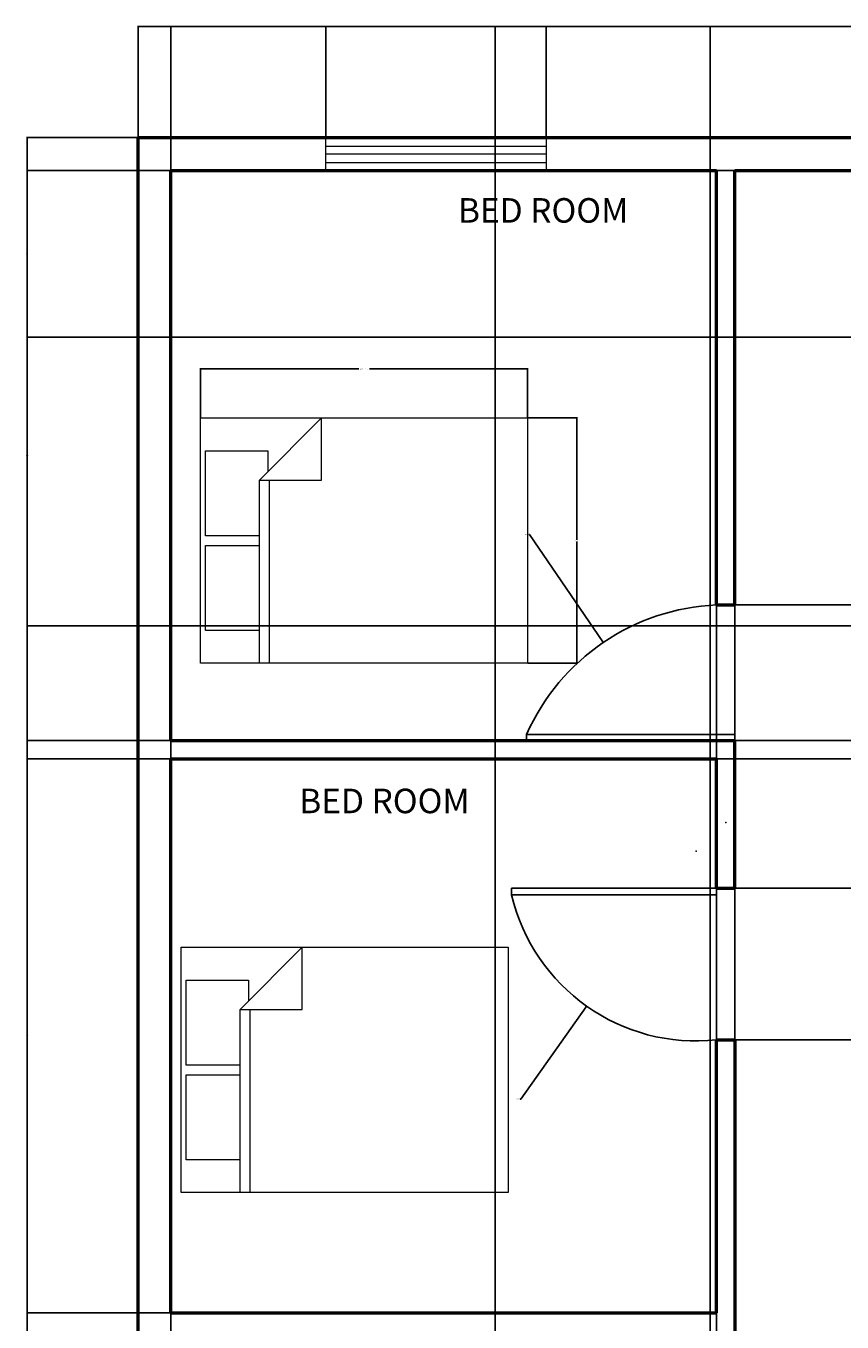
# Model space of a CAD drawing. Units: inches. Extents: x 2907 to 3328, y 1715 to 2286.
# Tile 3 of 5: x 2907 to 3107, y 1969 to 2286. Entities that reach past the tile are written whole.
import ezdxf

# ---------------------------------------------------------------- set-up
doc = ezdxf.new("R2010")
doc.units = ezdxf.units.IN
for name, color, linetype, lineweight in [('A-ANNO-DIMS', 2, 'Continuous', 18), ('A-AREA-IDEN', 7, 'Continuous', 25), ('A-DOOR', 3, 'Continuous', 25), ('A-FURN', 8, 'Continuous', 18), ('A-GLAZ', 4, 'Continuous', 18), ('A-WALL', 7, 'Continuous', 50)]:
    doc.layers.add(name, color=color, linetype=linetype, lineweight=lineweight)
doc.styles.get("Standard").update_dxf_attribs({"font": 'arial.ttf'})
doc.dimstyles.get("Standard").update_dxf_attribs({"dimtxt": 0.18, "dimasz": 0.18, "dimexe": 0.18, "dimexo": 0.0625, "dimgap": 0.09, "dimtad": 0, "dimtih": 1, "dimtoh": 1, "dimdec": 4, "dimzin": 0, "dimdsep": 46, "dimtxsty": 'Standard', "dimcen": 0.09, "dimadec": 0, "dimazin": 0, "dimtfac": 1, "dimtdec": 4, "dimtofl": 0, "dimtmove": 0, "dimatfit": 3, "dimfxl": 1, "dimtolj": 1, "dimtzin": 0, "dimarcsym": 0})

# ---------------------------------------------------------------- blocks, each defined once
blk = doc.blocks.new('Bed - Queen')
for p, q in [((0, -80.00003), (0, 0)), ((0, 0), (59.99999, 0)), ((59.99999, 0), (59.99999, -80.00003)), ((7.99999, -1.2), (28.79998, -1.2)), ((7.99999, -14.4), (7.99999, -1.2)), ((28.79998, -1.2), (28.79998, -14.4)), ((31.19999, -1.2), (51.99999, -1.2)), ((31.19999, -14.4), (31.19999, -1.2)), ((51.99999, -1.2), (51.99999, -16.4)), ((0, -14.4), (44.8, -14.4)), ((59.99999, -29.6), (44.8, -14.4)), ((44.8, -14.4), (44.8, -29.6)), ((44.8, -16.8), (0, -16.8)), ((51.99999, -16.4), (46.79936, -16.4)), ((44.8, -29.6), (59.99999, -29.6)), ((59.99999, -80.00003), (0, -80.00003))]:
    blk.add_line(p, q)
blk = doc.blocks.new('*D5')
at = {"layer": 'A-ANNO-DIMS', "color": 0, "lineweight": -2, "transparency": 16777216}
for p, q in [((2949.87, 2190.31), (2949.87, 2202.43)), ((2950.05, 2202.25), (2988.57, 2202.25)), ((3029.69, 2202.25), (2991.18, 2202.25)), ((3029.87, 2190.31), (3029.87, 2202.43))]:
    blk.add_line(p, q, dxfattribs=at)
at = {"layer": 'A-ANNO-DIMS', "color": 0, "transparency": 16777216}
for points in [[(2950.05, 2202.28), (2950.05, 2202.22), (2949.87, 2202.25)], [(3029.69, 2202.28), (3029.69, 2202.22), (3029.87, 2202.25)]]:
    blk.add_solid(points, dxfattribs=at)
at = {"layer": 'Defpoints', "color": 0, "transparency": 16777216}
for p in [(2949.87, 2202.25), (2949.87, 2190.25), (3029.87, 2190.25)]:
    blk.add_point(p, dxfattribs=at)
at = {"layer": 'A-ANNO-DIMS', "color": 0, "transparency": 16777216, "insert": (2989.87, 2202.25), "char_height": 0.18, "attachment_point": 5}
blk.add_mtext('\\A1;QUEEN BED 80 TYP.', dxfattribs=at)
blk = doc.blocks.new('*D6')
at = {"layer": 'A-ANNO-DIMS', "color": 0, "lineweight": -2, "transparency": 16777216}
for p, q in [((3029.94, 2190.25), (3042.05, 2190.25)), ((3041.87, 2190.07), (3041.87, 2160.43)), ((3041.87, 2130.43), (3041.87, 2160.07)), ((3029.94, 2130.25), (3042.05, 2130.25))]:
    blk.add_line(p, q, dxfattribs=at)
at = {"layer": 'A-ANNO-DIMS', "color": 0, "transparency": 16777216}
for points in [[(3041.84, 2190.07), (3041.9, 2190.07), (3041.87, 2190.25)], [(3041.84, 2130.43), (3041.9, 2130.43), (3041.87, 2130.25)]]:
    blk.add_solid(points, dxfattribs=at)
at = {"layer": 'Defpoints', "color": 0, "transparency": 16777216}
for p in [(3029.87, 2190.25), (3041.87, 2190.25), (3029.87, 2130.25)]:
    blk.add_point(p, dxfattribs=at)
at = {"layer": 'A-ANNO-DIMS', "color": 0, "transparency": 16777216, "insert": (3041.87, 2160.25), "char_height": 0.18, "attachment_point": 5}
blk.add_mtext('\\A1;60 TYP.', dxfattribs=at)
blk = doc.blocks.new('*D13')
at = {"layer": 'A-ANNO-DIMS', "color": 0, "lineweight": -2, "transparency": 16777216}
for p, q in [((2934.59, 2258.89), (2934.59, 2286.16)), ((3300.59, 2258.89), (3300.59, 2286.16)), ((2934.77, 2285.98), (3117.3, 2285.98)), ((3300.41, 2285.98), (3117.88, 2285.98))]:
    blk.add_line(p, q, dxfattribs=at)
at = {"layer": 'A-ANNO-DIMS', "color": 0, "transparency": 16777216}
for points in [[(2934.77, 2286.01), (2934.77, 2285.95), (2934.59, 2285.98)], [(3300.41, 2286.01), (3300.41, 2285.95), (3300.59, 2285.98)]]:
    blk.add_solid(points, dxfattribs=at)
at = {"layer": 'Defpoints', "color": 0, "transparency": 16777216}
for p in [(3300.59, 2285.98), (2934.59, 2258.83), (3300.59, 2258.83)]:
    blk.add_point(p, dxfattribs=at)
at = {"layer": 'A-ANNO-DIMS', "color": 0, "transparency": 16777216, "insert": (3117.59, 2285.98), "char_height": 0.18, "attachment_point": 5}
blk.add_mtext('\\A1;366', dxfattribs=at)
blk = doc.blocks.new('*D14')
at = {"layer": 'A-ANNO-DIMS', "color": 0, "lineweight": -2, "transparency": 16777216}
for p, q in [((2934.53, 2258.83), (2907.26, 2258.83)), ((2907.44, 2258.65), (2907.44, 2001.01)), ((2907.44, 1743.01), (2907.44, 2000.65)), ((2934.53, 1742.83), (2907.26, 1742.83))]:
    blk.add_line(p, q, dxfattribs=at)
at = {"layer": 'A-ANNO-DIMS', "color": 0, "transparency": 16777216}
for points in [[(2907.41, 2258.65), (2907.47, 2258.65), (2907.44, 2258.83)], [(2907.41, 1743.01), (2907.47, 1743.01), (2907.44, 1742.83)]]:
    blk.add_solid(points, dxfattribs=at)
at = {"layer": 'Defpoints', "color": 0, "transparency": 16777216}
for p in [(2907.44, 2258.83), (2934.59, 2258.83), (2934.59, 1742.83)]:
    blk.add_point(p, dxfattribs=at)
at = {"layer": 'A-ANNO-DIMS', "color": 0, "transparency": 16777216, "insert": (2907.44, 2000.83), "char_height": 0.18, "attachment_point": 5}
blk.add_mtext('\\A1;516', dxfattribs=at)
blk = doc.blocks.new('*D16')
at = {"layer": 'A-ANNO-DIMS', "color": 0, "lineweight": -2, "transparency": 16777216}
for p, q in [((2942.59, 2250.77), (2942.59, 1715.5)), ((3076.09, 2250.77), (3076.09, 1715.5)), ((2942.77, 1715.68), (3008.95, 1715.68)), ((3075.91, 1715.68), (3009.73, 1715.68))]:
    blk.add_line(p, q, dxfattribs=at)
at = {"layer": 'A-ANNO-DIMS', "color": 0, "transparency": 16777216}
for points in [[(2942.77, 1715.71), (2942.77, 1715.65), (2942.59, 1715.68)], [(3075.91, 1715.71), (3075.91, 1715.65), (3076.09, 1715.68)]]:
    blk.add_solid(points, dxfattribs=at)
at = {"layer": 'Defpoints', "color": 0, "transparency": 16777216}
for p in [(2942.59, 2250.83), (3076.09, 2250.83), (3076.09, 1715.68)]:
    blk.add_point(p, dxfattribs=at)
at = {"layer": 'A-ANNO-DIMS', "color": 0, "transparency": 16777216, "insert": (3009.34, 1715.68), "char_height": 0.18, "attachment_point": 5}
blk.add_mtext('\\A1;133.5', dxfattribs=at)
blk = doc.blocks.new('*D17')
at = {"layer": 'A-ANNO-DIMS', "color": 0, "lineweight": -2, "transparency": 16777216}
for p, q in [((3080.59, 2250.77), (3080.59, 1715.5)), ((3192.09, 2250.77), (3192.09, 1715.5)), ((3080.77, 1715.68), (3135.95, 1715.68)), ((3191.91, 1715.68), (3136.73, 1715.68))]:
    blk.add_line(p, q, dxfattribs=at)
at = {"layer": 'A-ANNO-DIMS', "color": 0, "transparency": 16777216}
for points in [[(3080.77, 1715.71), (3080.77, 1715.65), (3080.59, 1715.68)], [(3191.91, 1715.71), (3191.91, 1715.65), (3192.09, 1715.68)]]:
    blk.add_solid(points, dxfattribs=at)
at = {"layer": 'Defpoints', "color": 0, "transparency": 16777216}
for p in [(3080.59, 2250.83), (3192.09, 2250.83), (3192.09, 1715.68)]:
    blk.add_point(p, dxfattribs=at)
at = {"layer": 'A-ANNO-DIMS', "color": 0, "transparency": 16777216, "insert": (3136.34, 1715.68), "char_height": 0.18, "attachment_point": 5}
blk.add_mtext('\\A1;111.5', dxfattribs=at)
blk = doc.blocks.new('*D19')
at = {"layer": 'A-ANNO-DIMS', "color": 0, "lineweight": -2, "transparency": 16777216}
for p, q in [((2934.59, 2258.89), (2934.59, 2286.16)), ((2980.47, 2258.89), (2980.47, 2286.16)), ((2934.77, 2285.98), (2957.13, 2285.98)), ((2980.29, 2285.98), (2957.93, 2285.98))]:
    blk.add_line(p, q, dxfattribs=at)
at = {"layer": 'A-ANNO-DIMS', "color": 0, "transparency": 16777216}
for points in [[(2934.77, 2286.01), (2934.77, 2285.95), (2934.59, 2285.98)], [(2980.29, 2286.01), (2980.29, 2285.95), (2980.47, 2285.98)]]:
    blk.add_solid(points, dxfattribs=at)
at = {"layer": 'Defpoints', "color": 0, "transparency": 16777216}
for p in [(2980.47, 2285.98), (2934.59, 2258.83), (2980.47, 2258.83)]:
    blk.add_point(p, dxfattribs=at)
at = {"layer": 'A-ANNO-DIMS', "color": 0, "transparency": 16777216, "insert": (2957.53, 2285.98), "char_height": 0.18, "attachment_point": 5}
blk.add_mtext('\\A1;45.88', dxfattribs=at)
blk = doc.blocks.new('*D20')
at = {"layer": 'A-ANNO-DIMS', "color": 0, "lineweight": -2, "transparency": 16777216}
for p, q in [((2980.47, 2258.89), (2980.47, 2286.16)), ((3034.37, 2258.89), (3034.37, 2286.16)), ((2980.65, 2285.98), (3007.09, 2285.98)), ((3034.19, 2285.98), (3007.74, 2285.98))]:
    blk.add_line(p, q, dxfattribs=at)
at = {"layer": 'A-ANNO-DIMS', "color": 0, "transparency": 16777216}
for points in [[(2980.65, 2286.01), (2980.65, 2285.95), (2980.47, 2285.98)], [(3034.19, 2286.01), (3034.19, 2285.95), (3034.37, 2285.98)]]:
    blk.add_solid(points, dxfattribs=at)
at = {"layer": 'Defpoints', "color": 0, "transparency": 16777216}
for p in [(3034.37, 2285.98), (2980.47, 2258.83), (3034.37, 2258.83)]:
    blk.add_point(p, dxfattribs=at)
at = {"layer": 'A-ANNO-DIMS', "color": 0, "transparency": 16777216, "insert": (3007.42, 2285.98), "char_height": 0.18, "attachment_point": 5}
blk.add_mtext('\\A1;53.9', dxfattribs=at)
blk = doc.blocks.new('*D25')
at = {"layer": 'A-ANNO-DIMS', "color": 0, "lineweight": -2, "transparency": 16777216}
for p, q in [((2942.53, 2250.83), (2907.26, 2250.83)), ((2907.44, 2250.65), (2907.44, 2181.26)), ((2907.44, 2111.51), (2907.44, 2180.9)), ((2942.53, 2111.33), (2907.26, 2111.33))]:
    blk.add_line(p, q, dxfattribs=at)
at = {"layer": 'A-ANNO-DIMS', "color": 0, "transparency": 16777216}
for points in [[(2907.41, 2250.65), (2907.47, 2250.65), (2907.44, 2250.83)], [(2907.41, 2111.51), (2907.47, 2111.51), (2907.44, 2111.33)]]:
    blk.add_solid(points, dxfattribs=at)
at = {"layer": 'Defpoints', "color": 0, "transparency": 16777216}
for p in [(2907.44, 2250.83), (2942.59, 2250.83), (2942.59, 2111.33)]:
    blk.add_point(p, dxfattribs=at)
at = {"layer": 'A-ANNO-DIMS', "color": 0, "transparency": 16777216, "insert": (2907.44, 2181.08), "char_height": 0.18, "attachment_point": 5}
blk.add_mtext('\\A1;139.5', dxfattribs=at)
blk = doc.blocks.new('*D26')
at = {"layer": 'A-ANNO-DIMS', "color": 0, "lineweight": -2, "transparency": 16777216}
for p, q in [((2942.53, 2106.83), (2907.26, 2106.83)), ((2907.44, 2106.65), (2907.44, 2039.26)), ((2907.44, 1971.51), (2907.44, 2038.9)), ((2942.53, 1971.33), (2907.26, 1971.33))]:
    blk.add_line(p, q, dxfattribs=at)
at = {"layer": 'A-ANNO-DIMS', "color": 0, "transparency": 16777216}
for points in [[(2907.41, 2106.65), (2907.47, 2106.65), (2907.44, 2106.83)], [(2907.41, 1971.51), (2907.47, 1971.51), (2907.44, 1971.33)]]:
    blk.add_solid(points, dxfattribs=at)
at = {"layer": 'Defpoints', "color": 0, "transparency": 16777216}
for p in [(2907.44, 2106.83), (2942.59, 2106.83), (2942.59, 1971.33)]:
    blk.add_point(p, dxfattribs=at)
at = {"layer": 'A-ANNO-DIMS', "color": 0, "transparency": 16777216, "insert": (2907.44, 2039.08), "char_height": 0.18, "attachment_point": 5}
blk.add_mtext('\\A1;135.5', dxfattribs=at)
blk = doc.blocks.new('*D31')
at = {"layer": 'A-ANNO-DIMS', "color": 0, "lineweight": -2, "transparency": 16777216}
for p, q in [((2942.59, 1912.39), (2942.59, 2286.16)), ((3021.96, 1912.39), (3021.96, 2286.16)), ((2942.77, 2285.98), (2981.88, 2285.98)), ((3021.78, 2285.98), (2982.67, 2285.98))]:
    blk.add_line(p, q, dxfattribs=at)
at = {"layer": 'A-ANNO-DIMS', "color": 0, "transparency": 16777216}
for points in [[(2942.77, 2286.01), (2942.77, 2285.95), (2942.59, 2285.98)], [(3021.78, 2286.01), (3021.78, 2285.95), (3021.96, 2285.98)]]:
    blk.add_solid(points, dxfattribs=at)
at = {"layer": 'Defpoints', "color": 0, "transparency": 16777216}
for p in [(3021.96, 2285.98), (2942.59, 1912.33), (3021.96, 1912.33)]:
    blk.add_point(p, dxfattribs=at)
at = {"layer": 'A-ANNO-DIMS', "color": 0, "transparency": 16777216, "insert": (2982.27, 2285.98), "char_height": 0.18, "attachment_point": 5}
blk.add_mtext('\\A1;79.37', dxfattribs=at)
blk = doc.blocks.new('*D34')
at = {"layer": 'A-ANNO-DIMS', "color": 0, "lineweight": -2, "transparency": 16777216}
for p, q in [((3074.5, 1778.89), (3074.5, 2286.16)), ((3131.97, 1778.89), (3131.97, 2286.16)), ((3074.68, 2285.98), (3102.84, 2285.98)), ((3131.79, 2285.98), (3103.63, 2285.98))]:
    blk.add_line(p, q, dxfattribs=at)
at = {"layer": 'A-ANNO-DIMS', "color": 0, "transparency": 16777216}
for points in [[(3074.68, 2286.01), (3074.68, 2285.95), (3074.5, 2285.98)], [(3131.79, 2286.01), (3131.79, 2285.95), (3131.97, 2285.98)]]:
    blk.add_solid(points, dxfattribs=at)
at = {"layer": 'Defpoints', "color": 0, "transparency": 16777216}
for p in [(3131.97, 2285.98), (3074.5, 1778.83), (3131.97, 1778.83)]:
    blk.add_point(p, dxfattribs=at)
at = {"layer": 'A-ANNO-DIMS', "color": 0, "transparency": 16777216, "insert": (3103.24, 2285.98), "char_height": 0.18, "attachment_point": 5}
blk.add_mtext('\\A1;57.47', dxfattribs=at)
blk = doc.blocks.new('*D37')
at = {"layer": 'A-ANNO-DIMS', "color": 0, "lineweight": -2, "transparency": 16777216}
for p, q in [((3076.15, 2144.51), (3327.92, 2144.51)), ((3327.74, 2144.33), (3327.74, 2128.1)), ((3327.74, 2111.51), (3327.74, 2127.74)), ((3080.65, 2111.33), (3327.92, 2111.33))]:
    blk.add_line(p, q, dxfattribs=at)
at = {"layer": 'A-ANNO-DIMS', "color": 0, "transparency": 16777216}
for points in [[(3327.71, 2144.33), (3327.77, 2144.33), (3327.74, 2144.51)], [(3327.71, 2111.51), (3327.77, 2111.51), (3327.74, 2111.33)]]:
    blk.add_solid(points, dxfattribs=at)
at = {"layer": 'Defpoints', "color": 0, "transparency": 16777216}
for p in [(3076.09, 2144.51), (3327.74, 2144.51), (3080.59, 2111.33)]:
    blk.add_point(p, dxfattribs=at)
at = {"layer": 'A-ANNO-DIMS', "color": 0, "transparency": 16777216, "insert": (3327.74, 2127.92), "char_height": 0.18, "attachment_point": 5}
blk.add_mtext('\\A1;33.185', dxfattribs=at)
blk = doc.blocks.new('*D38')
at = {"layer": 'A-ANNO-DIMS', "color": 0, "lineweight": -2, "transparency": 16777216}
for p, q in [((3080.65, 2075.23), (3327.92, 2075.23)), ((3327.74, 2075.05), (3327.74, 2056.85)), ((3327.74, 2038.29), (3327.74, 2056.48)), ((3080.65, 2038.11), (3327.92, 2038.11))]:
    blk.add_line(p, q, dxfattribs=at)
at = {"layer": 'A-ANNO-DIMS', "color": 0, "transparency": 16777216}
for points in [[(3327.71, 2075.05), (3327.77, 2075.05), (3327.74, 2075.23)], [(3327.71, 2038.29), (3327.77, 2038.29), (3327.74, 2038.11)]]:
    blk.add_solid(points, dxfattribs=at)
at = {"layer": 'Defpoints', "color": 0, "transparency": 16777216}
for p in [(3080.59, 2075.23), (3327.74, 2075.23), (3080.59, 2038.11)]:
    blk.add_point(p, dxfattribs=at)
at = {"layer": 'A-ANNO-DIMS', "color": 0, "transparency": 16777216, "insert": (3327.74, 2056.67), "char_height": 0.18, "attachment_point": 5}
blk.add_mtext('\\A1;37.12', dxfattribs=at)
blk = doc.blocks.new('*D39')
at = {"layer": 'A-ANNO-DIMS', "color": 0, "lineweight": -2, "transparency": 16777216}
for p, q in [((3076.15, 2106.83), (3327.92, 2106.83)), ((3327.74, 2106.65), (3327.74, 2091.21)), ((3327.74, 2075.41), (3327.74, 2090.85)), ((3080.65, 2075.23), (3327.92, 2075.23))]:
    blk.add_line(p, q, dxfattribs=at)
at = {"layer": 'A-ANNO-DIMS', "color": 0, "transparency": 16777216}
for points in [[(3327.71, 2106.65), (3327.77, 2106.65), (3327.74, 2106.83)], [(3327.71, 2075.41), (3327.77, 2075.41), (3327.74, 2075.23)]]:
    blk.add_solid(points, dxfattribs=at)
at = {"layer": 'Defpoints', "color": 0, "transparency": 16777216}
for p in [(3076.09, 2106.83), (3327.74, 2106.83), (3080.59, 2075.23)]:
    blk.add_point(p, dxfattribs=at)
at = {"layer": 'A-ANNO-DIMS', "color": 0, "transparency": 16777216, "insert": (3327.74, 2091.03), "char_height": 0.18, "attachment_point": 5}
blk.add_mtext('\\A1;31.604', dxfattribs=at)
blk = doc.blocks.new('*D44')
at = {"layer": 'A-ANNO-DIMS', "color": 0, "lineweight": -2, "transparency": 16777216}
for p, q in [((3192.03, 2210.04), (2907.26, 2210.04)), ((2907.44, 2209.86), (2907.44, 2174.92)), ((2907.44, 2139.62), (2907.44, 2174.56)), ((3192.03, 2139.44), (2907.26, 2139.44))]:
    blk.add_line(p, q, dxfattribs=at)
at = {"layer": 'A-ANNO-DIMS', "color": 0, "transparency": 16777216}
for points in [[(2907.41, 2209.86), (2907.47, 2209.86), (2907.44, 2210.04)], [(2907.41, 2139.62), (2907.47, 2139.62), (2907.44, 2139.44)]]:
    blk.add_solid(points, dxfattribs=at)
at = {"layer": 'Defpoints', "color": 0, "transparency": 16777216}
for p in [(2907.44, 2210.04), (3192.09, 2210.04), (3192.09, 2139.44)]:
    blk.add_point(p, dxfattribs=at)
at = {"layer": 'A-ANNO-DIMS', "color": 0, "transparency": 16777216, "insert": (2907.44, 2174.74), "char_height": 0.18, "attachment_point": 5}
blk.add_mtext('\\A1;70.6', dxfattribs=at)
blk = doc.blocks.new('*D45')
at = {"layer": 'A-ANNO-DIMS', "color": 0, "lineweight": -2, "transparency": 16777216}
for p, q in [((3192.03, 2250.83), (2907.26, 2250.83)), ((2907.44, 2250.65), (2907.44, 2230.62)), ((2907.44, 2210.22), (2907.44, 2230.25)), ((3192.03, 2210.04), (2907.26, 2210.04))]:
    blk.add_line(p, q, dxfattribs=at)
at = {"layer": 'A-ANNO-DIMS', "color": 0, "transparency": 16777216}
for points in [[(2907.41, 2250.65), (2907.47, 2250.65), (2907.44, 2250.83)], [(2907.41, 2210.22), (2907.47, 2210.22), (2907.44, 2210.04)]]:
    blk.add_solid(points, dxfattribs=at)
at = {"layer": 'Defpoints', "color": 0, "transparency": 16777216}
for p in [(2907.44, 2250.83), (3192.09, 2250.83), (3192.09, 2210.04)]:
    blk.add_point(p, dxfattribs=at)
at = {"layer": 'A-ANNO-DIMS', "color": 0, "transparency": 16777216, "insert": (2907.44, 2230.43), "char_height": 0.18, "attachment_point": 5}
blk.add_mtext('\\A1;40.79', dxfattribs=at)
blk = doc.blocks.new('*D47')
at = {"layer": 'A-ANNO-DIMS', "color": 0, "lineweight": -2, "transparency": 16777216}
for p, q in [((3076.09, 2250.77), (3076.09, 1715.5)), ((3080.59, 2250.77), (3080.59, 1715.5)), ((3076.27, 1715.68), (3078.08, 1715.68)), ((3080.41, 1715.68), (3078.6, 1715.68))]:
    blk.add_line(p, q, dxfattribs=at)
at = {"layer": 'A-ANNO-DIMS', "color": 0, "transparency": 16777216}
for points in [[(3076.27, 1715.71), (3076.27, 1715.65), (3076.09, 1715.68)], [(3080.41, 1715.71), (3080.41, 1715.65), (3080.59, 1715.68)]]:
    blk.add_solid(points, dxfattribs=at)
at = {"layer": 'Defpoints', "color": 0, "transparency": 16777216}
for p in [(3076.09, 2250.83), (3080.59, 2250.83), (3080.59, 1715.68)]:
    blk.add_point(p, dxfattribs=at)
at = {"layer": 'A-ANNO-DIMS', "color": 0, "transparency": 16777216, "insert": (3078.34, 1715.68), "char_height": 0.18, "attachment_point": 5}
blk.add_mtext('\\A1;4.5', dxfattribs=at)
blk = doc.blocks.new('*D56')
at = {"layer": 'A-ANNO-DIMS', "color": 0, "lineweight": -2, "transparency": 16777216}
for p, q in [((2942.59, 1786.89), (2942.59, 2286.16)), ((3136.59, 1786.89), (3136.59, 2286.16)), ((2942.77, 2285.98), (3039.31, 2285.98)), ((3136.41, 2285.98), (3039.87, 2285.98))]:
    blk.add_line(p, q, dxfattribs=at)
at = {"layer": 'A-ANNO-DIMS', "color": 0, "transparency": 16777216}
for points in [[(2942.77, 2286.01), (2942.77, 2285.95), (2942.59, 2285.98)], [(3136.41, 2286.01), (3136.41, 2285.95), (3136.59, 2285.98)]]:
    blk.add_solid(points, dxfattribs=at)
at = {"layer": 'Defpoints', "color": 0, "transparency": 16777216}
for p in [(3136.59, 2285.98), (2942.59, 1786.83), (3136.59, 1786.83)]:
    blk.add_point(p, dxfattribs=at)
at = {"layer": 'A-ANNO-DIMS', "color": 0, "transparency": 16777216, "insert": (3039.59, 2285.98), "char_height": 0.18, "attachment_point": 5}
blk.add_mtext('\\A1;194', dxfattribs=at)
blk = doc.blocks.new('*D57')
at = {"layer": 'A-ANNO-DIMS', "color": 0, "lineweight": -2, "transparency": 16777216}
for p, q in [((3030.17, 2161.73), (3030.35, 2161.73)), ((3030.35, 2161.73), (3048.24, 2135.46)), ((3078.25, 2091.29), (3078.43, 2091.29)), ((3078.34, 2091.2), (3078.34, 2091.38))]:
    blk.add_line(p, q, dxfattribs=at)
at = {"layer": 'A-ANNO-DIMS', "color": 0, "transparency": 16777216}
blk.add_solid([(3048.27, 2135.48), (3048.22, 2135.45), (3048.34, 2135.31)], dxfattribs=at)
at = {"layer": 'Defpoints', "color": 0, "transparency": 16777216}
for p in [(3048.34, 2135.31), (3078.34, 2091.29)]:
    blk.add_point(p, dxfattribs=at)
at = {"layer": 'A-ANNO-DIMS', "color": 0, "transparency": 16777216, "insert": (3029.69, 2161.73), "char_height": 0.18, "attachment_point": 5}
blk.add_mtext('\\A1;R53.27', dxfattribs=at)
blk = doc.blocks.new('*D58')
at = {"layer": 'A-ANNO-DIMS', "color": 0, "lineweight": -2, "transparency": 16777216}
for p, q in [((3071.01, 2084.25), (3071.19, 2084.25)), ((3071.1, 2084.16), (3071.1, 2084.34)), ((3028.22, 2023.62), (3044.2, 2046.21)), ((3028.04, 2023.62), (3028.22, 2023.62))]:
    blk.add_line(p, q, dxfattribs=at)
at = {"layer": 'A-ANNO-DIMS', "color": 0, "transparency": 16777216}
blk.add_solid([(3044.17, 2046.23), (3044.22, 2046.19), (3044.3, 2046.36)], dxfattribs=at)
at = {"layer": 'Defpoints', "color": 0, "transparency": 16777216}
for p in [(3071.1, 2084.25), (3044.3, 2046.36)]:
    blk.add_point(p, dxfattribs=at)
at = {"layer": 'A-ANNO-DIMS', "color": 0, "transparency": 16777216, "insert": (3027.58, 2023.62), "char_height": 0.18, "attachment_point": 5}
blk.add_mtext('\\A1;R46.41', dxfattribs=at)

msp = doc.modelspace()

# ---------------------------------------------------------------- linework, layer by layer
at = {"layer": 'A-DOOR'}
for p, q in [((3080.5892, 2112.8572), (3029.63, 2112.8572)), ((3029.63, 2112.8572), (3029.63, 2111.3301)), ((3080.5892, 2111.3301), (3080.5892, 2112.8572)), ((3076.0892, 2075.2259), (3025.932, 2075.2259)), ((3025.932, 2075.2259), (3025.932, 2073.5769)), ((3076.0892, 2073.5769), (3076.0892, 2075.2259)), ((3025.932, 2073.5769), (3076.0892, 2073.5769))]:
    msp.add_line(p, q, dxfattribs=at)
for centre, radius, start, end in [((3078.3392, 2091.2935), 53.2689, 92.420808, 156.120891), ((3071.102, 2084.2537), 46.4146, 193.299003, 276.168317)]:
    msp.add_arc(centre, radius, start, end, dxfattribs=at)
at = {"layer": 'A-GLAZ'}
for p, q in [((2980.467, 2256.7847), (3034.3673, 2256.7168)), ((2980.467, 2254.8301), (3034.3673, 2254.8301)), ((2980.467, 2252.7736), (3034.3673, 2252.7736))]:
    msp.add_line(p, q, dxfattribs=at)
msp.add_lwpolyline([(2980.467, 2258.8301), (3034.3673, 2258.8301), (3034.3673, 2250.8301), (2980.467, 2250.8301)], close=True, dxfattribs=at)
at = {"layer": 'A-WALL'}
for p, q in [((2934.5892, 2258.8301), (3300.5892, 2258.8301)), ((2934.5892, 1778.8301), (2934.5892, 2258.8301)), ((2942.5892, 2250.8301), (3076.0892, 2250.8301)), ((2942.5892, 2111.3301), (2942.5892, 2250.8301)), ((3076.0892, 2144.5149), (3076.0892, 2250.8301)), ((3080.5892, 2144.5149), (3080.5892, 2250.8301)), ((3080.5892, 2250.8301), (3192.0892, 2250.8301)), ((3076.0892, 2144.5149), (3080.5892, 2144.5149)), ((2942.5892, 2111.3301), (3080.5892, 2111.3301)), ((3080.5892, 2075.2259), (3080.5892, 2111.3301)), ((2942.5892, 2106.8301), (3076.0892, 2106.8301)), ((2942.5892, 1971.3301), (2942.5892, 2106.8301)), ((3076.0892, 2075.2259), (3076.0892, 2106.8301)), ((3076.0892, 2075.2259), (3080.5892, 2075.2259)), ((3076.0892, 2038.1078), (3080.5892, 2038.1078)), ((3076.0892, 1971.3301), (3076.0892, 2038.1078)), ((3080.5892, 2038.1078), (3080.5892, 1966.8301)), ((2942.5892, 1971.3301), (3076.0892, 1971.3301))]:
    msp.add_line(p, q, dxfattribs=at)

# ---------------------------------------------------------------- block references
at = {"layer": 'A-FURN', "rotation": 90}
for p in [(2949.8744, 2130.2476), (2945.1432, 2000.7573)]:
    msp.add_blockref('Bed - Queen', p, dxfattribs=at)

# ---------------------------------------------------------------- texts
at = {"layer": 'A-AREA-IDEN', "char_height": 6, "attachment_point": 1}
for insert in [(3012.8352, 2244.0348), (2974.0149, 2099.5652)]:
    msp.add_mtext_dynamic_manual_height_columns('BED ROOM ', width=50.965346, gutter_width=12.5, heights=[0], dxfattribs=dict(at, insert=insert))

# ---------------------------------------------------------------- dimensions: what is measured, and where the dimension line sits
at = {"layer": 'A-ANNO-DIMS'}
for base, p1, p2, override, picture, middle in [((3300.5892, 2285.9816), (2934.5892, 2258.8301), (3300.5892, 2258.8301), {"dimdec": 0, "dimlfac": 1, "dimrnd": 0, "dimzin": 0, "dimdsep": 46, "dimlunit": 2}, '*D13', (3117.5892, 2285.9816)), ((2980.467, 2285.9816), (2934.5892, 2258.8301), (2980.467, 2258.8301), {"dimdec": 2, "dimlfac": 1, "dimrnd": 0, "dimzin": 0, "dimdsep": 46, "dimlunit": 2}, '*D19', (2957.5281, 2285.9816)), ((3021.96, 2285.9816), (2942.5892, 1912.3301), (3021.96, 1912.3301), {"dimdec": 2, "dimlfac": 1, "dimrnd": 0, "dimzin": 0, "dimdsep": 46, "dimlunit": 2}, '*D31', (2982.2746, 2285.9816)), ((3136.5892, 2285.9816), (2942.5892, 1786.8301), (3136.5892, 1786.8301), {"dimdec": 0, "dimlfac": 1, "dimrnd": 0, "dimzin": 0, "dimdsep": 46, "dimlunit": 2}, '*D56', (3039.5892, 2285.9816)), ((3034.3673, 2285.9816), (2980.467, 2258.8301), (3034.3673, 2258.8301), {"dimdec": 1, "dimlfac": 1, "dimrnd": 0, "dimzin": 0, "dimdsep": 46, "dimlunit": 2}, '*D20', (3007.4171, 2285.9816)), ((3131.9734, 2285.9816), (3074.499, 1778.8301), (3131.9734, 1778.8301), {"dimdec": 2, "dimlfac": 1, "dimrnd": 0, "dimzin": 0, "dimdsep": 46, "dimlunit": 2}, '*D34', (3103.2362, 2285.9816)), ((3076.0892, 1715.6786), (2942.5892, 2250.8301), (3076.0892, 2250.8301), {"dimdec": 1, "dimlfac": 1, "dimrnd": 0, "dimzin": 0, "dimdsep": 46, "dimlunit": 2}, '*D16', (3009.3392, 1715.6786)), ((3080.5892, 1715.6786), (3076.0892, 2250.8301), (3080.5892, 2250.8301), {"dimdec": 1, "dimlfac": 1, "dimrnd": 0, "dimzin": 0, "dimdsep": 46, "dimlunit": 2}, '*D47', (3078.3392, 1715.6786)), ((3192.0892, 1715.6786), (3080.5892, 2250.8301), (3192.0892, 2250.8301), {"dimdec": 1, "dimlfac": 1, "dimrnd": 0, "dimzin": 0, "dimdsep": 46, "dimlunit": 2}, '*D17', (3136.3392, 1715.6786))]:
    dim = msp.add_linear_dim(base=base, p1=p1, p2=p2, dimstyle='Standard', override=override, dxfattribs=at)
    dim.commit()
    dim.dimension.update_dxf_attribs({"geometry": picture, "text_midpoint": middle})
for base, p1, p2, override, picture, middle in [((2907.4377, 2258.8301), (2934.5892, 1742.8301), (2934.5892, 2258.8301), {"dimdec": 0, "dimlfac": 1, "dimrnd": 0, "dimzin": 0, "dimdsep": 46, "dimlunit": 2}, '*D14', (2907.4377, 2000.8301)), ((2907.4377, 2250.8301), (2942.5892, 2111.3301), (2942.5892, 2250.8301), {"dimdec": 1, "dimlfac": 1, "dimrnd": 0, "dimzin": 0, "dimdsep": 46, "dimlunit": 2}, '*D25', (2907.4377, 2181.0801)), ((2907.4377, 2250.8301), (3192.0892, 2210.0384), (3192.0892, 2250.8301), {"dimdec": 2, "dimlfac": 1, "dimrnd": 0, "dimzin": 0, "dimdsep": 46, "dimlunit": 2}, '*D45', (2907.4377, 2230.4342)), ((2907.4377, 2210.0384), (3192.0892, 2139.4387), (3192.0892, 2210.0384), {"dimdec": 1, "dimlfac": 1, "dimrnd": 0, "dimzin": 0, "dimdsep": 46, "dimlunit": 2}, '*D44', (2907.4377, 2174.7386)), ((3327.7407, 2144.5149), (3080.5892, 2111.3301), (3076.0892, 2144.5149), {"dimdec": 3, "dimlfac": 1, "dimrnd": 0, "dimzin": 0, "dimdsep": 46, "dimlunit": 2}, '*D37', (3327.7407, 2127.9225)), ((2907.4377, 2106.8301), (2942.5892, 1971.3301), (2942.5892, 2106.8301), {"dimdec": 1, "dimlfac": 1, "dimrnd": 0, "dimzin": 0, "dimdsep": 46, "dimlunit": 2}, '*D26', (2907.4377, 2039.0801)), ((3327.7407, 2106.8301), (3080.5892, 2075.2259), (3076.0892, 2106.8301), {"dimdec": 3, "dimlfac": 1, "dimrnd": 0, "dimzin": 0, "dimdsep": 46, "dimlunit": 2}, '*D39', (3327.7407, 2091.028)), ((3327.7407, 2075.2259), (3080.5892, 2038.1078), (3080.5892, 2075.2259), {"dimdec": 2, "dimlfac": 1, "dimrnd": 0, "dimzin": 0, "dimdsep": 46, "dimlunit": 2}, '*D38', (3327.7407, 2056.6669))]:
    dim = msp.add_linear_dim(base=base, p1=p1, p2=p2, angle=90, dimstyle='Standard', override=override, dxfattribs=at)
    dim.commit()
    dim.dimension.update_dxf_attribs({"geometry": picture, "text_midpoint": middle})
for base, p1, p2, angle, text, picture, middle in [((2949.8744, 2202.2476), (3029.8745, 2190.2476), (2949.8744, 2190.2476), 180, 'QUEEN BED <> TYP.', '*D5', (2989.8744, 2202.2476)), ((3041.8745, 2190.2476), (3029.8745, 2130.2476), (3029.8745, 2190.2476), 90, '<> TYP.', '*D6', (3041.8745, 2160.2476))]:
    dim = msp.add_linear_dim(base=base, p1=p1, p2=p2, angle=angle, text=text, dimstyle='Standard', override={"dimdec": 0, "dimlfac": 1, "dimrnd": 0, "dimzin": 0, "dimdsep": 46, "dimlunit": 2}, dxfattribs=at)
    dim.commit()
    dim.dimension.update_dxf_attribs({"geometry": picture, "text_midpoint": middle})
for center, mpoint, picture, middle in [((3078.3392, 2091.2935), (3048.343, 2135.314), '*D57', (3029.6854, 2161.7264)), ((3071.102, 2084.2537), (3044.3032, 2046.3573), '*D58', (3027.5815, 2023.6194))]:
    dim = msp.add_radius_dim(center=center, mpoint=mpoint, dimstyle='Standard', override={"dimdec": 2, "dimlfac": 1, "dimrnd": 0, "dimzin": 0, "dimdsep": 46, "dimlunit": 2}, dxfattribs=at)
    dim.commit()
    dim.dimension.update_dxf_attribs({"geometry": picture, "text_midpoint": middle, "dimtype": 164})

doc.saveas('drawing.dxf')
